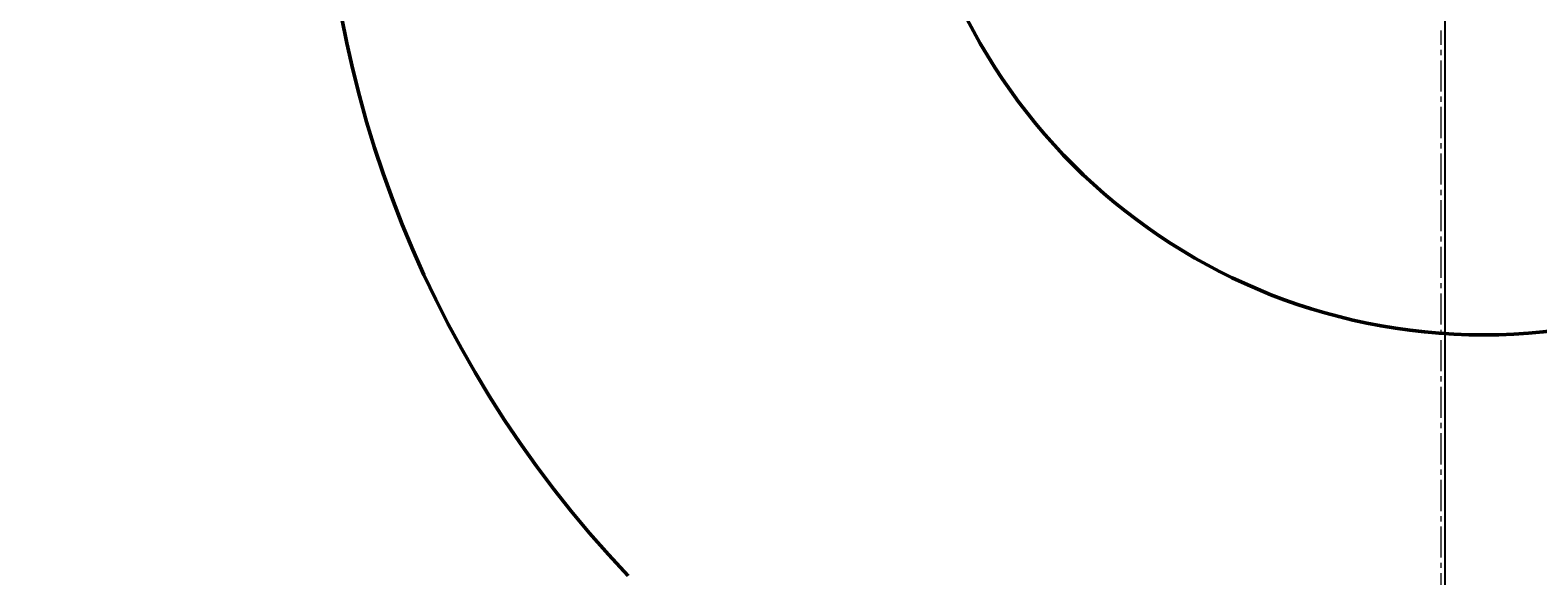
# Model space of a CAD drawing. Units: millimetres. Extents: x -60 to 113, y -37 to 126.
# Tile 12 of 17: x -23 to 13, y 70 to 83. Entities that reach past the tile are written whole.
import ezdxf

# ---------------------------------------------------------------- set-up
doc = ezdxf.new("R2010")
doc.units = ezdxf.units.MM
doc.header["$MEASUREMENT"] = 0
doc.linetypes.add('CENTER2', pattern=[1.125, 0.75, -0.125, 0.125, -0.125])
for name, color, linetype, lineweight in [('M-CNTR', 4, 'CENTER2', 18), ('M-DIMS', 2, 'Continuous', 25), ('M-OUTL', 7, 'Continuous', 50)]:
    doc.layers.add(name, color=color, linetype=linetype, lineweight=lineweight)
doc.styles.get("Standard").update_dxf_attribs({"font": 'arial.ttf'})
doc.dimstyles.get("Standard").update_dxf_attribs({"dimtxt": 0.18, "dimasz": 0.18, "dimexe": 0.18, "dimexo": 0.0625, "dimgap": 0.09, "dimtad": 0, "dimtih": 1, "dimtoh": 1, "dimdec": 4, "dimzin": 0, "dimdsep": 46, "dimtxsty": 'Standard', "dimcen": 0.09, "dimadec": 0, "dimazin": 0, "dimtfac": 1, "dimtdec": 4, "dimtofl": 0, "dimtmove": 0, "dimatfit": 3, "dimfxl": 1, "dimtolj": 1, "dimtzin": 0, "dimarcsym": 0})

# ---------------------------------------------------------------- blocks, each defined once
blk = doc.blocks.new('*U1')
at = {"layer": 'M-CNTR', "color": 0, "transparency": 16777216}
blk.add_line((0, -27.12), (0, -5.4), dxfattribs=at)
blk = doc.blocks.new('*D7')
at = {"layer": 'Defpoints', "color": 0, "transparency": 16777216}
for p in [(48.606, 76.822), (-30.775, 49.351)]:
    blk.add_point(p, dxfattribs=at)
at = {"layer": 'M-DIMS', "color": 0, "lineweight": -2, "transparency": 16777216}
for p, q in [((37.821, 73.09), (48.435, 76.764)), ((37.641, 73.09), (37.821, 73.09))]:
    blk.add_line(p, q, dxfattribs=at)
at = {"layer": 'M-DIMS', "color": 0, "transparency": 16777216}
blk.add_solid([(48.426, 76.792), (48.445, 76.735), (48.606, 76.822)], dxfattribs=at)
at = {"layer": 'M-DIMS', "color": 0, "transparency": 16777216, "insert": (35.165, 73.09), "char_height": 0.18, "attachment_point": 5}
blk.add_mtext('\\A1;{\\H11.11111x;R84}', dxfattribs=at)
blk = doc.blocks.new('*D12')
at = {"layer": 'Defpoints', "color": 0, "transparency": 16777216}
for p in [(10.532, 88.533), (-58.719, 6.903), (11.329, 6.903)]:
    blk.add_point(p, dxfattribs=at)
at = {"layer": 'M-DIMS', "color": 0, "lineweight": -2, "transparency": 16777216}
for p, q in [((10.47, 88.533), (-58.899, 88.533)), ((-58.719, 88.353), (-58.719, 48.829)), ((-58.719, 7.083), (-58.719, 46.607)), ((11.267, 6.903), (-58.899, 6.903))]:
    blk.add_line(p, q, dxfattribs=at)
at = {"layer": 'M-DIMS', "color": 0, "transparency": 16777216}
for points in [[(-58.749, 88.353), (-58.689, 88.353), (-58.719, 88.533)], [(-58.749, 7.083), (-58.689, 7.083), (-58.719, 6.903)]]:
    blk.add_solid(points, dxfattribs=at)
at = {"layer": 'M-DIMS', "color": 0, "transparency": 16777216, "insert": (-58.719, 47.718), "char_height": 0.18, "attachment_point": 5}
blk.add_mtext('\\A1;{\\H11.11111x;82}', dxfattribs=at)
blk = doc.blocks.new('*D16')
at = {"layer": 'Defpoints', "color": 0, "transparency": 16777216}
for p in [(10.712, 88.533), (10.712, 88.533), (10.712, 6.442)]:
    blk.add_point(p, dxfattribs=at)
at = {"layer": 'M-DIMS', "color": 0, "lineweight": -2, "transparency": 16777216}
for p, q in [((10.712, 88.47), (10.712, 6.262)), ((10.712, 88.47), (10.712, 6.262)), ((10.532, 6.442), (10.352, 6.442)), ((10.892, 6.442), (11.072, 6.442))]:
    blk.add_line(p, q, dxfattribs=at)
at = {"layer": 'M-DIMS', "color": 0, "transparency": 16777216}
for points in [[(10.532, 6.472), (10.532, 6.412), (10.712, 6.442)], [(10.892, 6.472), (10.892, 6.412), (10.712, 6.442)]]:
    blk.add_solid(points, dxfattribs=at)
at = {"layer": 'M-DIMS', "color": 0, "transparency": 16777216, "insert": (11.536, 6.442), "char_height": 0.18, "attachment_point": 5}
blk.add_mtext('\\A1;0.0000', dxfattribs=at)
blk = doc.blocks.new('*D17')
at = {"layer": 'Defpoints', "color": 0, "transparency": 16777216}
for p in [(67.355, 124.823), (10.532, 88.533), (67.355, 6.442)]:
    blk.add_point(p, dxfattribs=at)
at = {"layer": 'M-DIMS', "color": 0, "lineweight": -2, "transparency": 16777216}
for p, q in [((10.532, 88.595), (10.532, 125.003)), ((10.712, 124.823), (37.422, 124.823)), ((67.175, 124.823), (40.465, 124.823)), ((67.355, 6.504), (67.355, 125.003))]:
    blk.add_line(p, q, dxfattribs=at)
at = {"layer": 'M-DIMS', "color": 0, "transparency": 16777216}
for points in [[(10.712, 124.853), (10.712, 124.793), (10.532, 124.823)], [(67.175, 124.853), (67.175, 124.793), (67.355, 124.823)]]:
    blk.add_solid(points, dxfattribs=at)
at = {"layer": 'M-DIMS', "color": 0, "transparency": 16777216, "insert": (38.944, 124.823), "char_height": 0.18, "attachment_point": 5}
blk.add_mtext('\\A1;{\\H11.11111x;56}', dxfattribs=at)
blk = doc.blocks.new('HOLE-D28')
blk.add_circle((14, 14), 14)
blk = doc.blocks.new('*D24')
at = {"layer": 'Defpoints', "color": 0, "transparency": 16777216}
for p in [(48.596, 76.851), (-30.775, 49.351)]:
    blk.add_point(p, dxfattribs=at)
at = {"layer": 'M-DIMS', "color": 0, "lineweight": -2, "transparency": 16777216}
for p, q in [((96.218, 93.35), (48.766, 76.909)), ((96.398, 93.35), (96.218, 93.35)), ((-30.865, 49.351), (-30.685, 49.351)), ((-30.775, 49.261), (-30.775, 49.441))]:
    blk.add_line(p, q, dxfattribs=at)
at = {"layer": 'M-DIMS', "color": 0, "transparency": 16777216}
blk.add_solid([(48.756, 76.938), (48.776, 76.881), (48.596, 76.851)], dxfattribs=at)
at = {"layer": 'M-DIMS', "color": 0, "transparency": 16777216, "insert": (97.018, 93.35), "char_height": 0.18, "attachment_point": 5}
blk.add_mtext('\\A1;R84.0000', dxfattribs=at)

msp = doc.modelspace()

# ---------------------------------------------------------------- linework, layer by layer
at = {"layer": 'M-OUTL'}
msp.add_arc((10.62227, 88.53289), 27, 43.425324, 223.425324, dxfattribs=at)

# ---------------------------------------------------------------- block references
at = {"layer": 'M-CNTR'}
msp.add_blockref('*U1', (10.62227, 88.53289), dxfattribs=at)
at = {"layer": 'M-OUTL'}
msp.add_blockref('HOLE-D28', (-2.3502, 75.7872), dxfattribs=at)

# ---------------------------------------------------------------- dimensions: what is measured, and where the dimension line sits
at = {"layer": 'M-DIMS'}
dim = msp.add_linear_dim(base=(67.35481, 124.82251), p1=(10.53227, 88.53289), p2=(67.35481, 6.44179), text='{\\H11.11111x;56}', dimstyle='Standard', override={"dimclrd": 0, "dimclre": 0, "dimclrt": 0}, dxfattribs=at)
dim.commit()
dim.dimension.update_dxf_attribs({"geometry": '*D17', "text_midpoint": (38.94354, 124.82251)})
dim = msp.add_radius_dim(center=(-30.77517, 49.3506), mpoint=(48.59582, 76.85052), dimstyle='Standard', override={"dimdec": 4, "dimlfac": 1, "dimrnd": 0, "dimzin": 0, "dimdsep": 46, "dimlunit": 2}, dxfattribs=at)
dim.commit()
dim.dimension.update_dxf_attribs({"geometry": '*D24', "text_midpoint": (97.01779, 93.35047), "dimtype": 164})
dim = msp.add_linear_dim(base=(-58.71857, 6.9027), p1=(10.53227, 88.53289), p2=(11.32938, 6.9027), angle=90, text='{\\H11.11111x;82}', dimstyle='Standard', override={"dimclrd": 0, "dimclre": 0, "dimclrt": 0}, dxfattribs=at)
dim.commit()
dim.dimension.update_dxf_attribs({"geometry": '*D12', "text_midpoint": (-58.71857, 47.71779)})
dim = msp.add_linear_dim(base=(10.712269814, 6.441792179), p1=(10.712269814, 88.5328900903), p2=(10.712269814, 88.5328900903), dimstyle='Standard', override={"dimclrd": 0, "dimclre": 0, "dimclrt": 0}, dxfattribs=at)
dim.commit()
dim.dimension.update_dxf_attribs({"geometry": '*D16', "text_midpoint": (11.5355917785, 6.441792179)})
dim = msp.add_radius_dim(center=(-30.77517, 49.3506), mpoint=(48.60556, 76.82239), text='{\\H11.11111x;R84}', dimstyle='Standard', override={"dimclrd": 0, "dimclre": 0, "dimclrt": 0}, dxfattribs=at)
dim.commit()
dim.dimension.update_dxf_attribs({"geometry": '*D7', "text_midpoint": (35.16548, 73.09007), "dimtype": 164})

doc.saveas('drawing.dxf')
